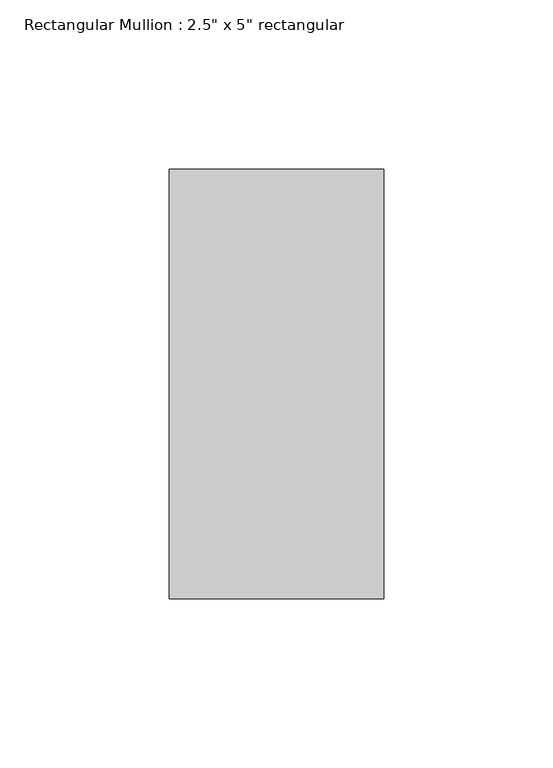
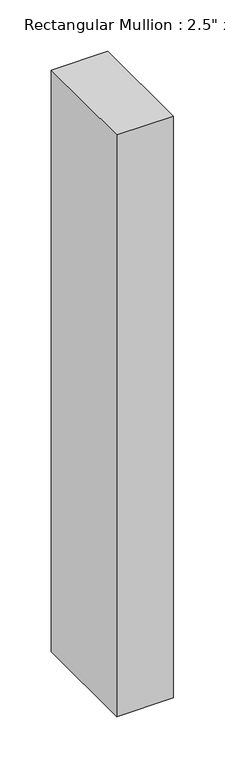
"""IFC4 building model written with IfcOpenShell, lengths in millimetres: member geometry."""

from ifc_helpers import new_model, si_unit, frame, origin, place, context, project, spatial, polyline, outline, extrude, source, transform, mapped, element, save


def member_106f6fb5(model_context):
    return source(origin(), model_context, "Body", "SweptSolid", [
        extrude(outline(polyline([(31.75, 63.5), (31.75, -63.5), (-31.75, -63.5), (-31.75, 63.5), (31.75, 63.5)])), frame((0.0, 0.0, -690.6281505), z_axis=(0.0, 0.0, 1.0), x_axis=(1.0, 0.0, 0.0)), (0.0, 0.0, 1.0), 690.6281505),
    ])


if __name__ == "__main__":
    model = new_model("IFC4")
    model_context = context("Model", 3, world=origin())
    ifc_project = project(units=[si_unit("LENGTHUNIT", "METRE", prefix="MILLI")], contexts=[model_context])
    site = spatial("IfcSite", under=ifc_project)
    building = spatial("IfcBuilding", under=site)
    placement = place(None, origin())
    member_shape = member_106f6fb5(model_context)
    element("IfcMember", 1, ObjectType="Rectangular Mullion : 2.5\" x 5\" rectangular", at=placement, inside=building, context=model_context, shape_type="MappedRepresentation", body=[
        mapped(member_shape, transform((0.0, 0.0, 0.0), x_axis=(1.0, 0.0, 0.0), y_axis=(0.0, 1.0, 0.0), z_axis=(0.0, 0.0, 1.0))),
    ])
    save(model, "model.ifc")

# Revit data of these elements
# Type "Rectangular Mullion : 2.5\" x 5\" rectangular"
#   built-in parameter 1007304 = 0.416667 (stored number, unit not read)
#   built-in parameter 1007301 = 0.104167 (stored number, unit not read)
#   built-in parameter 1007300 = 0.104167 (stored number, unit not read)
# Element 1 (IfcMember, "Rectangular Mullion : 2.5\" x 5\" rectangular")
#   Materials on its faces: "Aluminum"
# Materials
#   "Aluminum": class "Metal", colour RGB 247 247 247, transparency 0, Description = "Aluminum 6061", Cost = 0
